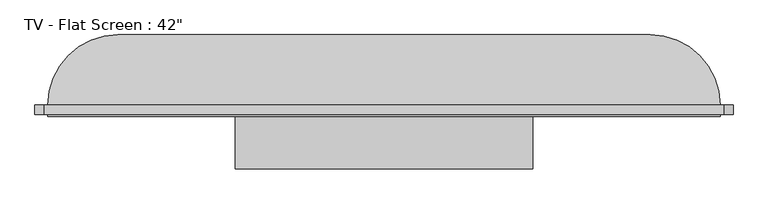
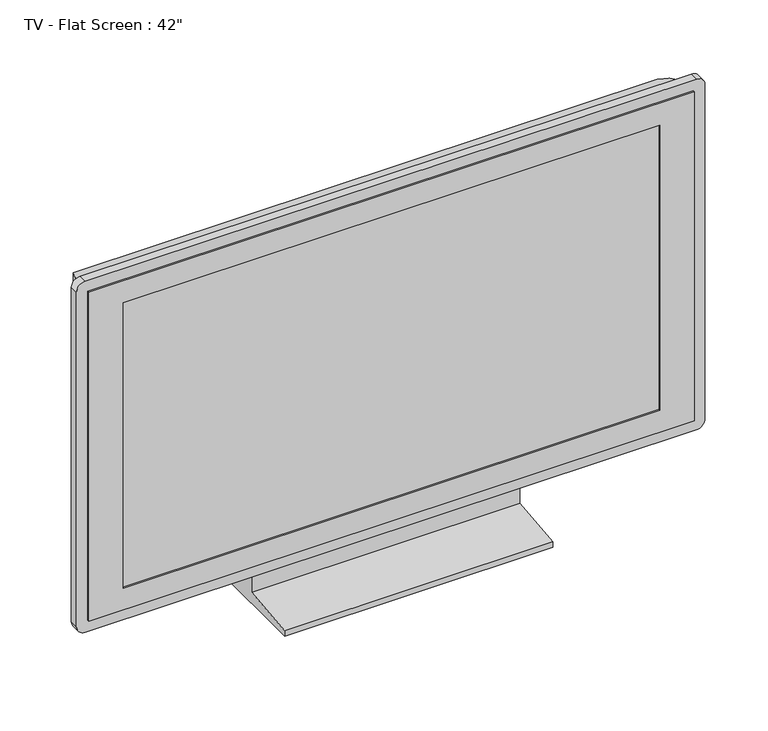
"""IFC4 building model written with IfcOpenShell, lengths in millimetres: furniture geometry."""

from ifc_helpers import new_model, si_unit, point, frame, frame_2d, origin, place, context, project, spatial, polyline, circle_curve, ellipse_curve, trimmed, segment, composite_curve, outline, extrude, faceted_brep, source, transform, mapped, element, save
from ifc_brep_helpers import plane_surface, cylinder_surface, advanced_brep


def furniture_7a3aaa4f(model_context):
    return source(origin(), model_context, "Body", "SolidModel", [
        extrude(outline(polyline([(-51.4613764, 80.0), (-1.4613764, 80.0), (48.5386236, 0.0), (-151.4613764, 0.0), (-151.4613764, 10.0), (-51.4613764, 20.0), (-51.4613764, 80.0)])), frame((-237.0858282, 0.0, 0.0), z_axis=(1.0, 0.0, 0.0), x_axis=(0.0, 1.0, 0.0)), (0.0, 0.0, 1.0), 466.2826281),
        faceted_brep([(522.338114, -69.4613764, 684.6160909), (-530.2271423, -69.4613764, 684.6160909), (-530.2271423, -69.4613764, 80.0), (522.338114, -69.4613764, 80.0), (-470.2271423, -69.4613764, 644.6160909), (462.338114, -69.4613764, 644.6160909), (462.338114, -69.4613764, 120.0), (-470.2271423, -69.4613764, 120.0), (522.338114, -51.4613764, 684.6160909), (522.338114, -51.4613764, 80.0), (-530.2271423, -51.4613764, 80.0), (-530.2271423, -51.4613764, 684.6160909), (-470.2271423, -66.4613764, 644.6160909), (-470.2271423, -66.4613764, 120.0), (462.338114, -66.4613764, 120.0), (462.338114, -66.4613764, 644.6160909)], [[[0, 1, 2, 3], [4, 5, 6, 7]], [[8, 9, 10, 11]], [[1, 0, 8, 11]], [[2, 1, 11, 10]], [[3, 2, 10, 9]], [[0, 3, 9, 8]], [[12, 13, 14, 15]], [[12, 15, 5, 4]], [[15, 14, 6, 5]], [[14, 13, 7, 6]], [[13, 12, 4, 7]]]),
        extrude(outline(composite_curve([segment(polyline([(704.6160909, 527.338114), (704.6160909, -535.2271423)]), True, "CONTINUOUS"), segment(trimmed(circle_curve(frame_2d((689.6160909, -535.2271423)), 15.0), [point((704.6160909, -535.2271423))], [point((689.6160909, -550.2271423))], False, "CARTESIAN"), True, "CONTINUOUS"), segment(polyline([(689.6160909, -550.2271423), (75.0, -550.2271423)]), True, "CONTINUOUS"), segment(trimmed(circle_curve(frame_2d((75.0, -535.2271423)), 15.0), [point((75.0, -550.2271423))], [point((60.0, -535.2271423))], False, "CARTESIAN"), True, "CONTINUOUS"), segment(polyline([(60.0, -535.2271423), (60.0, 527.338114)]), True, "CONTINUOUS"), segment(trimmed(circle_curve(frame_2d((75.0, 527.338114)), 15.0), [point((60.0, 527.338114))], [point((75.0, 542.338114))], False, "CARTESIAN"), True, "CONTINUOUS"), segment(polyline([(75.0, 542.338114), (689.6160909, 542.338114)]), True, "CONTINUOUS"), segment(trimmed(circle_curve(frame_2d((689.6160909, 527.338114)), 15.0), [point((689.6160909, 542.338114))], [point((704.6160909, 527.338114))], False, "CARTESIAN"), True, "CONTINUOUS")], self_intersect=False), holes=[polyline([(684.6160909, 522.338114), (80.0, 522.338114), (80.0, -530.2271423), (684.6160909, -530.2271423), (684.6160909, 522.338114)])]), frame((0.0, -66.4613764, 0.0), z_axis=(0.0, 1.0, 0.0), x_axis=(0.0, 0.0, 1.0)), (0.0, 0.0, 1.0), 15.0),
        advanced_brep(
        [(-530.2271423, -51.4613764, 80.0), (522.338114, -51.4613764, 80.0), (522.338114, -51.4613764, 684.6160909), (-530.2271423, -51.4613764, 684.6160909), (412.338114, 58.5386236, 80.0), (-420.2271423, 58.5386236, 80.0), (-420.2271423, 58.5386236, 574.6160909), (412.338114, 58.5386236, 574.6160909)],
        [
            (0, 1),
            (1, 2),
            (2, 3),
            (3, 0),
            (4, 5),
            (5, 6),
            (6, 7),
            (7, 4),
            (0, 5, circle_curve(frame((-420.2271423, -51.4613764, 80.0), z_axis=(0.0, 0.0, -1.0), x_axis=(-1.0, 0.0, 0.0)), 110.0)),
            (4, 1, circle_curve(frame((412.338114, -51.4613764, 80.0), z_axis=(0.0, 0.0, -1.0), x_axis=(1.0, 0.0, 0.0)), 110.0)),
            (7, 2, ellipse_curve(frame((412.338114, -51.4613764, 574.6160909), z_axis=(0.7071067811865475, 0.0, -0.7071067811865475), x_axis=(0.7071067811865474, 0.0, 0.7071067811865476)), 155.5634919, 110.0)),
            (6, 3, ellipse_curve(frame((-420.2271423, -51.4613764, 574.6160909), z_axis=(0.7071067811865475, 0.0, 0.7071067811865475), x_axis=(-0.7071067811865476, 0.0, 0.7071067811865474)), 155.5634919, 110.0)),
        ],
        [
            plane_surface(frame((-530.2271423, -51.4613764, 684.6160909), z_axis=(0.0, -1.0, 0.0), x_axis=(-1.0, 0.0, 0.0))),
            plane_surface(frame((-530.2271423, 58.5386236, 684.6160909), z_axis=(0.0, 1.0, 0.0), x_axis=(1.0, 0.0, 0.0))),
            plane_surface(frame((-530.2271423, -51.4613764, 80.0), z_axis=(0.0, 0.0, -1.0), x_axis=(0.0, 1.0, 0.0))),
            cylinder_surface(frame((412.338114, -51.4613764, 80.0), z_axis=(0.0, 0.0, 1.0), x_axis=(1.0, 0.0, 0.0)), 110.0),
            cylinder_surface(frame((522.338114, -51.4613764, 574.6160909), z_axis=(-1.0, 0.0, 0.0), x_axis=(0.0, 0.0, 1.0)), 110.0),
            cylinder_surface(frame((-420.2271423, -51.4613764, 684.6160909), z_axis=(0.0, 0.0, -1.0), x_axis=(-1.0, 0.0, 0.0)), 110.0),
        ],
        [
            (0, [[1, 2, 3, 4]]),
            (1, [[5, 6, 7, 8]]),
            (2, [[-1, 9, -5, 10]]),
            (3, [[11, -2, -10, -8]]),
            (4, [[-11, -7, 12, -3]]),
            (5, [[-12, -6, -9, -4]]),
        ],
    ),
    ])


if __name__ == "__main__":
    model = new_model("IFC4")
    model_context = context("Model", 3, world=origin())
    ifc_project = project(units=[si_unit("LENGTHUNIT", "METRE", prefix="MILLI")], contexts=[model_context])
    site = spatial("IfcSite", under=ifc_project)
    building = spatial("IfcBuilding", under=site)
    placement = place(None, origin())
    furniture_shape = furniture_7a3aaa4f(model_context)
    element("IfcFurniture", 1, ObjectType="TV - Flat Screen : 42\"", at=placement, inside=building, context=model_context, shape_type="MappedRepresentation", body=[
        mapped(furniture_shape, transform((0.0, 0.0, 0.0), x_axis=(1.0, 0.0, 0.0), y_axis=(0.0, 1.0, 0.0), z_axis=(0.0, 0.0, 1.0))),
    ])
    save(model, "model.ifc")

# Revit data of these elements
# Type "TV - Flat Screen : 42\""
#   SinAng = 0' - 0.0193"
#   L = 3' - 0.71517"
#   H = 1' - 8.65418"
#   Thickness = 0' - 4.33071"
#   Diagonal = 3' - 6.12598"
#   CosAng = 0' - 0.03431"
#   Stand [instance default] = yes
#   Default Elevation = 0
# Element 1 (IfcFurniture, "TV - Flat Screen : 42\"")
#   Materials on its faces: "TV - Black", "TV - Glass", "TV - Screen"
# Materials
#   "TV - Black": colour RGB 49 49 49, transparency 0
#   "TV - Glass": colour RGB 157 157 157, transparency 0.9
#   "TV - Screen": colour RGB 0 0 0, transparency 0
